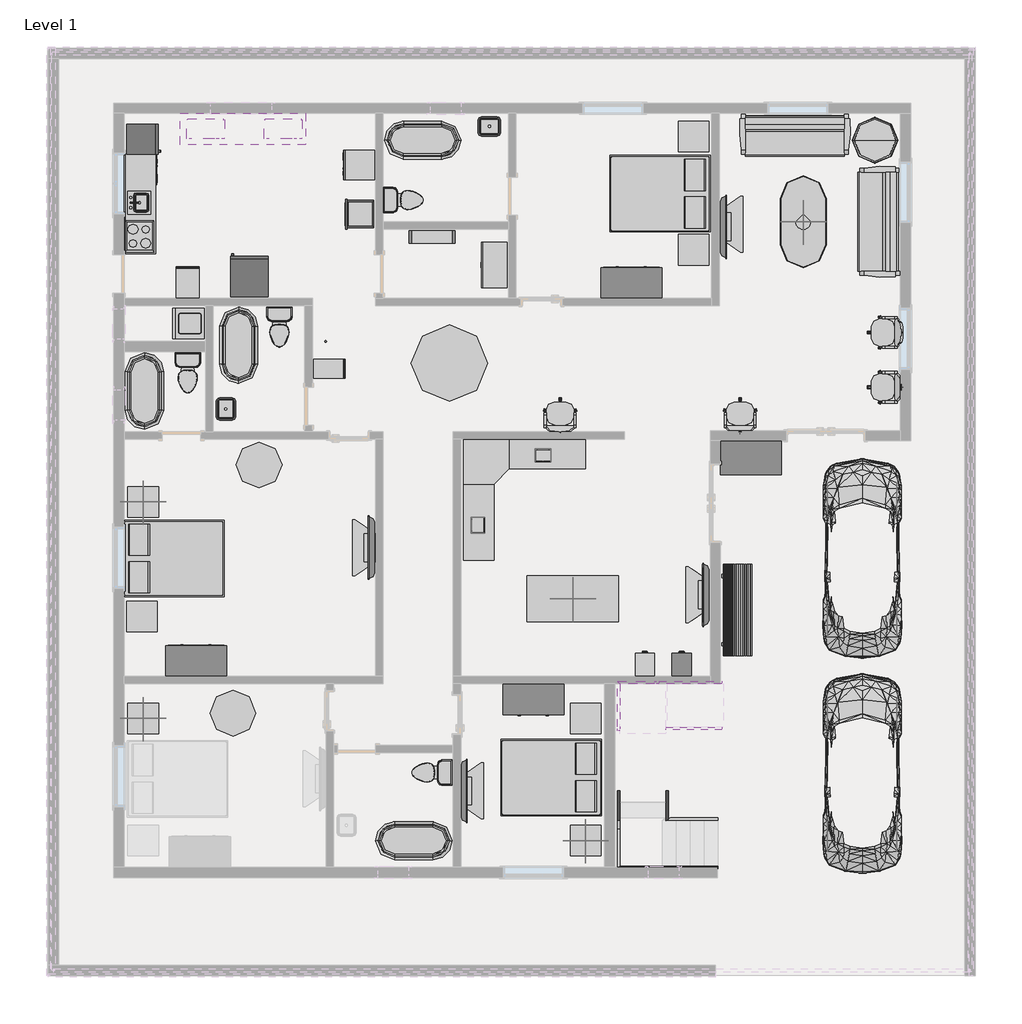
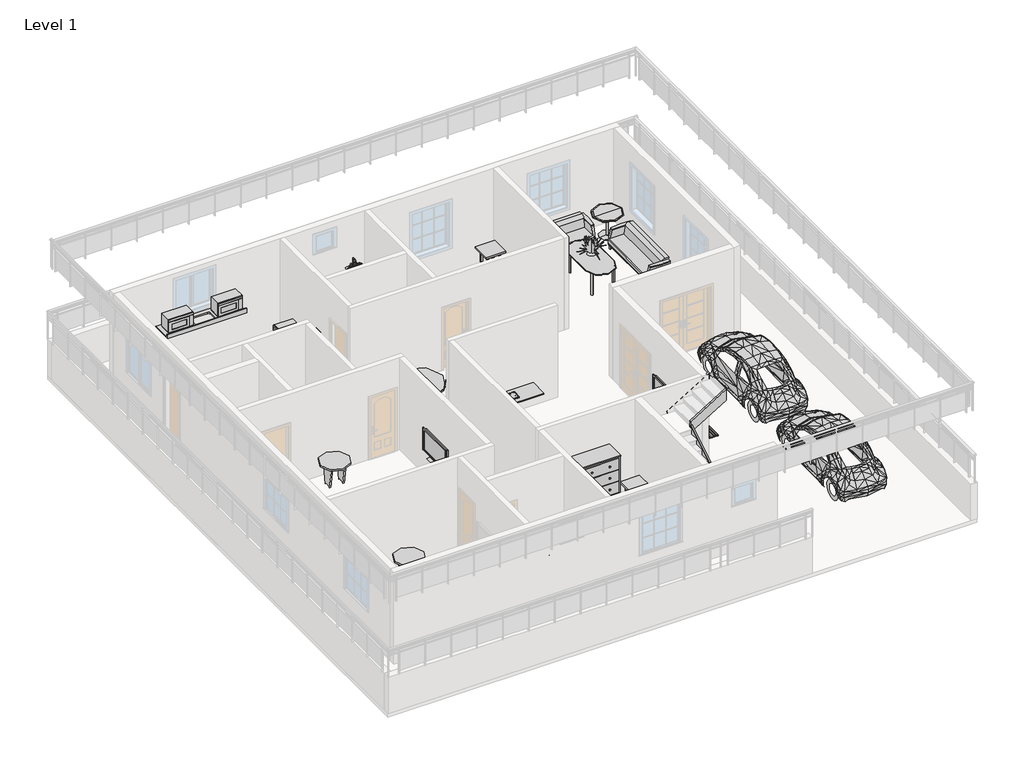
# One storey, part 6 of 6: 41 furniture elements, 16 proxies, 12 flow terminals, 10 members, 6 geographic elements.
# Revit data of these elements (continued)
# Elements 41, 42, 43 (IfcFurniture, "Dresser : 48\" x 72\" x 24\"") (continued)
#   Materials on its faces: "Laminate, Ivory, Matte", "Cherry", "Laminate - Ivory, Glossy"
# Element 44 (IfcFurniture, "Entertainment Center : 72\" x 72\" x 24\"")
#   Phase Created = New Construction
#   Materials on its faces: "Steel, Chrome Plated", "Glass - Clear, Grey"
# Element 45 (IfcFurniture, "Shelving : 36\" x 10\" x 72\"")
#   Phase Created = New Construction
#   Materials on its faces: "Birch"
# Elements 46, 47 (IfcFurniture, "Sofa-Pensi : 84\"")
#   Phase Created = New Construction
#   Materials on its faces: "Cherry", "Linen, Beige", "Steel, Chrome Plated"
# Element 48 (IfcFurniture, "Storage Pedestal : 20\" x 36\" x 36\"")
#   Phase Created = New Construction
#   Materials on its faces: "Steel, Paint Finish, Ivory, Glossy", "Steel, Chrome Plated"
# Elements 49, 50, 51, 52 (IfcFurniture, "TV - Flat Screen : 50\"")
#   Stand = yes
#   Phase Created = New Construction
#   Materials on its faces: "TV - Black", "TV - Glass", "TV - Screen"
# Elements 53, 54, 55, 56 (IfcFurniture, "TV Stand : TV Stand")
#   Phase Created = New Construction
#   Materials on its faces: "Melamine - Gray", "Glass - Shelves"
# Element 57 (IfcFurniture, "Table-Dining : 24\" x 36\" x 24\"")
#   Phase Created = New Construction
#   Materials on its faces: "Steel, Chrome Plated", "Glass - Clear, Grey"
# Element 58 (IfcFurniture, "Table-Dining Oval : 36\" x 72\"")
#   Phase Created = New Construction
#   Materials on its faces: "Steel, Chrome Plated", "Glass - Clear, Grey"
# Element 59 (IfcFurniture, "Table-Dining Round w Chairs : 60\" Diameter")
#   Phase Created = New Construction
#   Materials on its faces: "Pine", "Laminate, Linen, Matte"
# Elements 60, 61 (IfcFurniture, "Table-Ellipse : 72\" x 36\"")
#   Phase Created = New Construction
#   Materials on its faces: "Birch", "Laminate - Black"
# Elements 62, 63, 64, 65, 66, 67, 68 (IfcFurniture, "Table-Night Stand : 24\" x 24\" x 30\"")
#   Phase Created = New Construction
#   Materials on its faces: "Birch", "Laminate, Ivory, Matte"
# Element 69 (IfcFurniture, "Table-Round : 36\" Diameter")
#   Phase Created = New Construction
#   Materials on its faces: "Steel, Chrome Plated", "Birch"
# Element 70 (IfcGeographicElement, "Park Bench : 72\"")
#   Phase Created = New Construction
#   Materials on its faces: "Wood - Teak", "Steel, Paint Finish, Dark Gray, Matte"
# Elements 71, 72, 73, 74, 75 (IfcGeographicElement, "RPC Plant - Tropical : Agave - 1.5'")
#   Phase Created = New Construction
# Elements 76, 77, 78, 79, 80, 81, 82, 83, 84, 85 (IfcMember, "Stringer - 2\" Width")
#   Phase Created = New Construction
# Materials
#   "Plastic, Opaque Black": class "Plastic", colour RGB 0 0 0, transparency 0.7, Description = "Plastic, generic, opaque black", Cost = 0
#   "Steel, Paint Finish, Ivory, Matte": class "Metal", colour RGB 247 247 239, transparency 0, Description = "Steel, paint finish, ivory, matte", Cost = 0
#   "Steel, Chrome Plated": class "Metal", colour RGB 17 17 17, transparency 0, Description = "Chromiuim plated steel", Cost = 0
#   "Steel, Polished": class "Metal", colour RGB 57 57 57, transparency 0, Description = "Polished steel", Cost = 0
#   "Steel, Paint Finish, Ivory, Glossy": class "Metal", colour RGB 247 247 239, transparency 0, Description = "Steel, paint finish, ivory, glossy", Cost = 0
#   "Cabinets": colour RGB 249 249 249, transparency 0
#   "Cabinets - Handles": class "Metal", colour RGB 57 57 57, transparency 0
#   "Laminate, Ivory, Matte": class "Plastic", colour RGB 247 247 239, transparency 0, Description = "Plastic Laminate - Ivory, Matte", Cost = 0
#   "Metal - Stainless Steel, Polished": class "Metal", colour RGB 216 216 216, transparency 0
#   "Porcelain, Linen": class "Ceramic", colour RGB 249 239 230, transparency 0, Description = "Porcelain, linen", Cost = 0
#   "Laminate, Linen, Matte": class "Plastic", colour RGB 249 239 230, transparency 0, Description = "Plastic Laminate - Linen, Matte", Cost = 0
#   "Porcelain, Ivory": class "Ceramic", colour RGB 247 247 239, transparency 0, Description = "Porcelain, ivory", Cost = 0
#   "Birch": class "Wood", colour RGB 224 178 126, transparency 0, Description = "Betula Alleghaniensis", Cost = 0
#   "Linen, White": class "Textile", colour RGB 247 247 239, transparency 0, Description = "Linen, white", Cost = 0
#   "Textile - Slate Blue": class "Fabric", colour RGB 98 102 118, transparency 0
#   "Laminate - Ivory, Glossy": colour RGB 247 247 239, transparency 0
#   "Cherry": class "Wood", colour RGB 226 177 128, transparency 0, Description = "Prunus Serotina", Cost = 0
#   "Linen, Beige": class "Textile", colour RGB 249 239 230, transparency 0, Description = "Linen, beige", Cost = 0
#   "Melamine - Gray": class "Wood", colour RGB 49 49 49, transparency 0
#   "Glass - Clear, Grey": class "Glass", colour RGB 252 255 255, transparency 0.64
#   "Pine": class "Wood", colour RGB 223 192 134, transparency 0, Description = "Pinus Echinata", Cost = 0
#   "Laminate - Black": colour RGB 0 0 0, transparency 0
#   "Wood - Teak": class "Wood", colour RGB 120 73 19, transparency 0
#   "Steel, Paint Finish, Dark Gray, Matte": class "Metal", colour RGB 98 98 98, transparency 0, Description = "Steel, paint finish, dark gray, matte", Cost = 0
#   "Glass": class "Glass", colour RGB 0 128 192, transparency 0.75, Description = "Soda Lime Glass", Cost = 0
#   "Steel": class "Metal", colour RGB 247 247 247, transparency 0, Description = "Steel, mill finish", Cost = 0
#   "Counter Top": class "Wood", colour RGB 226 177 128, transparency 0
#   "TV - Black": colour RGB 49 49 49, transparency 0
#   "TV - Glass": colour RGB 157 157 157, transparency 0.9
#   "TV - Screen": colour RGB 0 0 0, transparency 0
#   "Glass - Shelves": class "Glass", colour RGB 167 167 167, transparency 0.9
